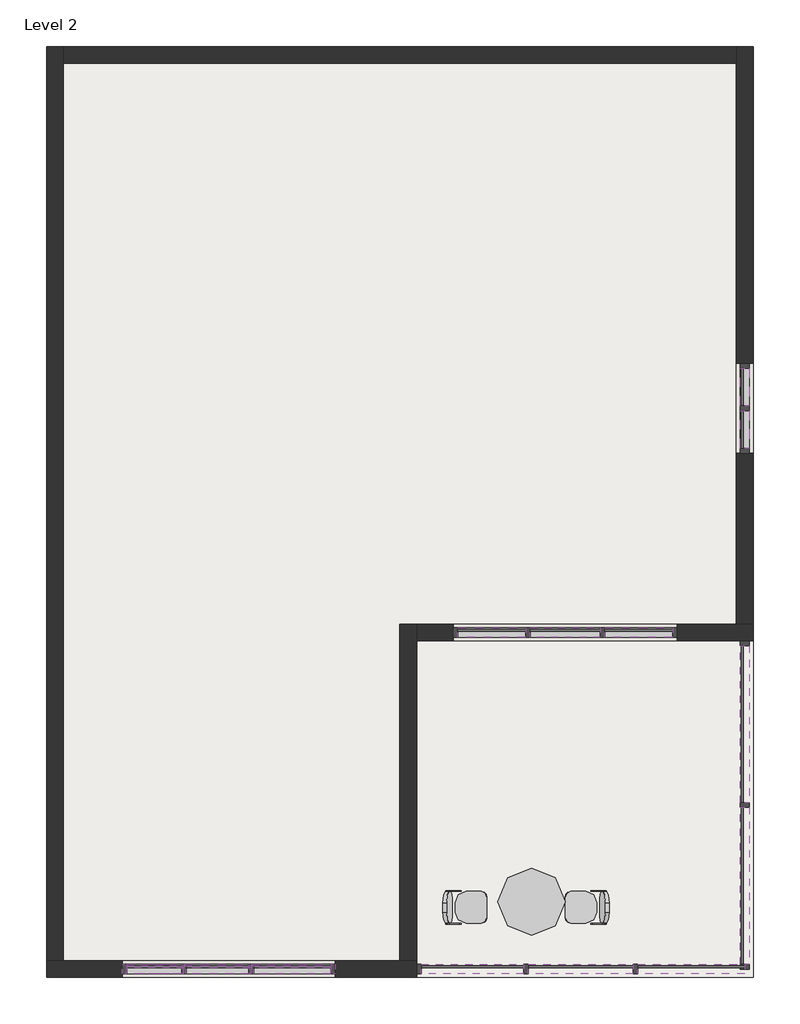
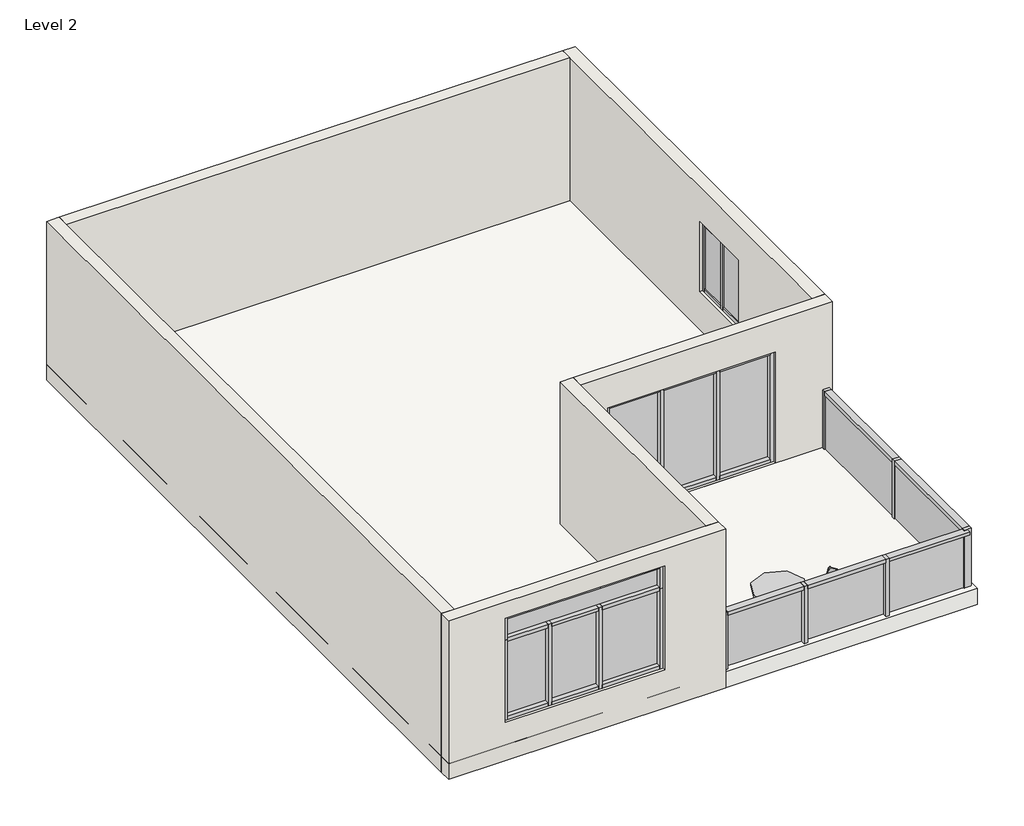
# One storey: 46 members, 14 plates, 6 walls, 3 furniture elements, 1 roof.
"""IFC4 building model written with IfcOpenShell, lengths in millimetres."""

from ifc_helpers import new_model, si_unit, frame, origin, place, context, project, spatial, polyline, outline, extrude, faceted_brep, transform, mapped, element, save
from components import furniture_eb3a3c23, furniture_ec754799, member_194e59d8, member_ff82125d, member_73c23c35, member_972adede, member_15823cb3, member_7b995701, member_7db1855a, member_7297827b, member_d2e7e466, member_3a0a7659, member_811bfb9a, member_697f972d, member_74e81316, member_78934672, member_cad56782, member_3e830f4e, member_0b7646a3, member_57611c17, member_d1dfe9dc, member_a36b500a, member_3bd69304, member_36d9a658, member_194437a1, member_a139046c, member_0767621a, member_3374d9b6, member_53538a1b, system_panel_glazed_d02f90d0, system_panel_glazed_14014958, system_panel_glazed_c1b5d4b5, system_panel_glazed_28e33a90, system_panel_glazed_a47c5a86, system_panel_glazed_f6d699fe, system_panel_glazed_2d65dcb0, system_panel_glazed_5a84bc76, system_panel_glazed_73858ddd, system_panel_glazed_ae745dbd, system_panel_glazed_f31d7781

model = new_model("IFC4")

# Units and contexts
model_context = context("Model", 3, world=origin())
ifc_project = project(units=[si_unit("LENGTHUNIT", "METRE", prefix="MILLI")], contexts=[model_context])

# Site, building, storey
site = spatial("IfcSite", under=ifc_project)
building = spatial("IfcBuilding", under=site)
storey = spatial("IfcBuildingStorey", under=building, Name="Level 2", Elevation=3048.0)

# Furniture
placement = place(None, origin())
furniture_shape = furniture_eb3a3c23(model_context)
element("IfcFurniture", 1, ObjectType="Seating-Auditorium : 18\" x 24\" x 30\"", at=placement, inside=storey, context=model_context, shape_type="MappedRepresentation", body=[
    mapped(furniture_shape, transform((-7671.1776869, -12175.0861758, 3048.0), x_axis=(0.0, 1.0, 0.0), y_axis=(-1.0, 0.0, 0.0), z_axis=(0.0, 0.0, 1.0))),
])
element("IfcFurniture", 2, ObjectType="Seating-Auditorium : 18\" x 24\" x 30\"", at=placement, inside=storey, context=model_context, shape_type="MappedRepresentation", body=[
    mapped(furniture_shape, transform((-9727.3285066, -11853.6304381, 3048.0), x_axis=(0.0, -1.0, 0.0), y_axis=(1.0, 0.0, 0.0), z_axis=(0.0, 0.0, 1.0))),
])
furniture_2_shape = furniture_ec754799(model_context)
element("IfcFurniture", 3, ObjectType="Table-Dining Round : 36\" Diameter", at=placement, inside=storey, context=model_context, shape_type="MappedRepresentation", body=[
    mapped(furniture_2_shape, transform((-8726.735064, -11753.2796184, 3048.0), x_axis=(1.0, 0.0, 0.0), y_axis=(0.0, 1.0, 0.0), z_axis=(0.0, 0.0, 1.0))),
])

# Members
member_shape = member_194e59d8(model_context)
element("IfcMember", 4, ObjectType="Rectangular Mullion : 2.5\" x 5\" rectangular", at=placement, inside=storey, context=model_context, shape_type="MappedRepresentation", body=[
    mapped(member_shape, transform((-7689.6030968, -8280.558307, 5481.9310998), x_axis=(0.0, 0.0, 1.0), y_axis=(0.0, -1.0, 0.0), z_axis=(1.0, 0.0, 0.0))),
])
member_2_shape = member_ff82125d(model_context)
element("IfcMember", 5, ObjectType="Rectangular Mullion : 2.5\" x 5\" rectangular", at=placement, inside=storey, context=model_context, shape_type="MappedRepresentation", body=[
    mapped(member_2_shape, transform((-8705.6030968, -8280.558307, 5481.9310998), x_axis=(0.0, 0.0, 1.0), y_axis=(0.0, -1.0, 0.0), z_axis=(1.0, 0.0, 0.0))),
])
element("IfcMember", 6, ObjectType="Rectangular Mullion : 2.5\" x 5\" rectangular", at=placement, inside=storey, context=model_context, shape_type="MappedRepresentation", body=[
    mapped(member_2_shape, transform((-6705.3530968, -8280.558307, 5481.9310998), x_axis=(0.0, 0.0, 1.0), y_axis=(0.0, -1.0, 0.0), z_axis=(1.0, 0.0, 0.0))),
])
element("IfcMember", 7, ObjectType="Rectangular Mullion : 2.5\" x 5\" rectangular", at=placement, inside=storey, context=model_context, shape_type="MappedRepresentation", body=[
    mapped(member_shape, transform((-8642.1030968, -8280.558307, 3352.8), x_axis=(0.0, 0.0, -1.0), y_axis=(0.0, -1.0, 0.0), z_axis=(-1.0, 0.0, 0.0))),
])
element("IfcMember", 8, ObjectType="Rectangular Mullion : 2.5\" x 5\" rectangular", at=placement, inside=storey, context=model_context, shape_type="MappedRepresentation", body=[
    mapped(member_2_shape, transform((-7626.1030968, -8280.558307, 3352.8), x_axis=(0.0, 0.0, -1.0), y_axis=(0.0, -1.0, 0.0), z_axis=(-1.0, 0.0, 0.0))),
])
element("IfcMember", 9, ObjectType="Rectangular Mullion : 2.5\" x 5\" rectangular", at=placement, inside=storey, context=model_context, shape_type="MappedRepresentation", body=[
    mapped(member_2_shape, transform((-9626.3530968, -8280.558307, 3352.8), x_axis=(0.0, 0.0, -1.0), y_axis=(0.0, -1.0, 0.0), z_axis=(-1.0, 0.0, 0.0))),
])
member_3_shape = member_73c23c35(model_context)
element("IfcMember", 10, ObjectType="Rectangular Mullion : 2.5\" x 5\" rectangular", at=placement, inside=storey, context=model_context, shape_type="MappedRepresentation", body=[
    mapped(member_3_shape, transform((-12433.0530968, -12852.558307, 5780.2418911), x_axis=(0.0, 0.0, 1.0), y_axis=(0.0, -1.0, 0.0), z_axis=(1.0, 0.0, 0.0))),
])
member_4_shape = member_972adede(model_context)
element("IfcMember", 11, ObjectType="Rectangular Mullion : 2.5\" x 5\" rectangular", at=placement, inside=storey, context=model_context, shape_type="MappedRepresentation", body=[
    mapped(member_4_shape, transform((-13347.4530968, -12852.558307, 5780.2418911), x_axis=(0.0, 0.0, 1.0), y_axis=(0.0, -1.0, 0.0), z_axis=(1.0, 0.0, 0.0))),
])
member_5_shape = member_15823cb3(model_context)
element("IfcMember", 12, ObjectType="Rectangular Mullion : 2.5\" x 5\" rectangular", at=placement, inside=storey, context=model_context, shape_type="MappedRepresentation", body=[
    mapped(member_5_shape, transform((-14185.6530968, -12852.558307, 5780.2418911), x_axis=(-1.0, 0.0, 0.0), y_axis=(0.0, -1.0, 0.0), z_axis=(0.0, 0.0, 1.0))),
])
member_6_shape = member_7b995701(model_context)
element("IfcMember", 13, ObjectType="Rectangular Mullion : 2.5\" x 5\" rectangular", at=placement, inside=storey, context=model_context, shape_type="MappedRepresentation", body=[
    mapped(member_6_shape, transform((-13379.2030968, -12852.558307, 5323.0418911), x_axis=(0.0, 0.0, 1.0), y_axis=(0.0, -1.0, 0.0), z_axis=(1.0, 0.0, 0.0))),
])
member_7_shape = member_7db1855a(model_context)
element("IfcMember", 14, ObjectType="Rectangular Mullion : 2.5\" x 5\" rectangular", at=placement, inside=storey, context=model_context, shape_type="MappedRepresentation", body=[
    mapped(member_7_shape, transform((-12464.8030968, -12852.558307, 5323.0418911), x_axis=(0.0, 0.0, 1.0), y_axis=(0.0, -1.0, 0.0), z_axis=(1.0, 0.0, 0.0))),
])
member_8_shape = member_7297827b(model_context)
element("IfcMember", 15, ObjectType="Rectangular Mullion : 2.5\" x 5\" rectangular", at=placement, inside=storey, context=model_context, shape_type="MappedRepresentation", body=[
    mapped(member_8_shape, transform((-13347.4530968, -12852.558307, 3783.7672722), x_axis=(1.0, 0.0, 0.0), y_axis=(0.0, -1.0, 0.0), z_axis=(0.0, 0.0, -1.0))),
])
element("IfcMember", 16, ObjectType="Rectangular Mullion : 2.5\" x 5\" rectangular", at=placement, inside=storey, context=model_context, shape_type="MappedRepresentation", body=[
    mapped(member_8_shape, transform((-12433.0530968, -12852.558307, 3783.7672722), x_axis=(1.0, 0.0, 0.0), y_axis=(0.0, -1.0, 0.0), z_axis=(0.0, 0.0, -1.0))),
])
member_9_shape = member_d2e7e466(model_context)
element("IfcMember", 17, ObjectType="Rectangular Mullion : 2.5\" x 5\" rectangular", at=placement, inside=storey, context=model_context, shape_type="MappedRepresentation", body=[
    mapped(member_9_shape, transform((-13315.7030968, -12852.558307, 3783.7672722), x_axis=(0.0, 0.0, -1.0), y_axis=(0.0, -1.0, 0.0), z_axis=(-1.0, 0.0, 0.0))),
])
member_10_shape = member_3a0a7659(model_context)
element("IfcMember", 18, ObjectType="Rectangular Mullion : 2.5\" x 5\" rectangular", at=placement, inside=storey, context=model_context, shape_type="MappedRepresentation", body=[
    mapped(member_10_shape, transform((-14122.1530968, -12852.558307, 3783.7672722), x_axis=(0.0, 0.0, -1.0), y_axis=(0.0, -1.0, 0.0), z_axis=(-1.0, 0.0, 0.0))),
])
member_11_shape = member_811bfb9a(model_context)
element("IfcMember", 19, ObjectType="Rectangular Mullion : 2.5\" x 5\" rectangular", at=placement, inside=storey, context=model_context, shape_type="MappedRepresentation", body=[
    mapped(member_11_shape, transform((-14185.6530968, -12852.558307, 5323.0418911), x_axis=(-1.0, 0.0, 0.0), y_axis=(0.0, -1.0, 0.0), z_axis=(0.0, 0.0, 1.0))),
])
member_12_shape = member_697f972d(model_context)
element("IfcMember", 20, ObjectType="Rectangular Mullion : 2.5\" x 5\" rectangular", at=placement, inside=storey, context=model_context, shape_type="MappedRepresentation", body=[
    mapped(member_12_shape, transform((-11353.5530968, -12852.558307, 5323.0418911), x_axis=(0.0, 0.0, 1.0), y_axis=(0.0, -1.0, 0.0), z_axis=(1.0, 0.0, 0.0))),
])
member_13_shape = member_74e81316(model_context)
element("IfcMember", 21, ObjectType="Rectangular Mullion : 2.5\" x 5\" rectangular", at=placement, inside=storey, context=model_context, shape_type="MappedRepresentation", body=[
    mapped(member_13_shape, transform((-11353.5530968, -12852.558307, 5780.2418911), x_axis=(0.0, 0.0, 1.0), y_axis=(0.0, -1.0, 0.0), z_axis=(1.0, 0.0, 0.0))),
])
member_14_shape = member_78934672(model_context)
element("IfcMember", 22, ObjectType="Rectangular Mullion : 2.5\" x 5\" rectangular", at=placement, inside=storey, context=model_context, shape_type="MappedRepresentation", body=[
    mapped(member_14_shape, transform((-12401.3030968, -12852.558307, 3783.7672722), x_axis=(0.0, 0.0, -1.0), y_axis=(0.0, -1.0, 0.0), z_axis=(-1.0, 0.0, 0.0))),
])
element("IfcMember", 23, ObjectType="Rectangular Mullion : 2.5\" x 5\" rectangular", at=placement, inside=storey, context=model_context, shape_type="MappedRepresentation", body=[
    mapped(member_5_shape, transform((-11290.0530968, -12852.558307, 5323.0418911), x_axis=(1.0, 0.0, 0.0), y_axis=(0.0, -1.0, 0.0), z_axis=(0.0, 0.0, -1.0))),
])
element("IfcMember", 24, ObjectType="Rectangular Mullion : 2.5\" x 5\" rectangular", at=placement, inside=storey, context=model_context, shape_type="MappedRepresentation", body=[
    mapped(member_11_shape, transform((-11290.0530968, -12852.558307, 3783.7672722), x_axis=(1.0, 0.0, 0.0), y_axis=(0.0, -1.0, 0.0), z_axis=(0.0, 0.0, -1.0))),
])
member_15_shape = member_cad56782(model_context)
element("IfcMember", 25, ObjectType="Rectangular Mullion : 2.5\" x 5\" rectangular", at=placement, inside=storey, context=model_context, shape_type="MappedRepresentation", body=[
    mapped(member_15_shape, transform((-8673.8530968, -8280.558307, 3352.8), x_axis=(1.0, 0.0, 0.0), y_axis=(0.0, -1.0, 0.0), z_axis=(0.0, 0.0, -1.0))),
])
element("IfcMember", 26, ObjectType="Rectangular Mullion : 2.5\" x 5\" rectangular", at=placement, inside=storey, context=model_context, shape_type="MappedRepresentation", body=[
    mapped(member_15_shape, transform((-7657.8530968, -8280.558307, 3352.8), x_axis=(1.0, 0.0, 0.0), y_axis=(0.0, -1.0, 0.0), z_axis=(0.0, 0.0, -1.0))),
])
member_16_shape = member_3e830f4e(model_context)
element("IfcMember", 27, ObjectType="Rectangular Mullion : 2.5\" x 5\" rectangular", at=placement, inside=storey, context=model_context, shape_type="MappedRepresentation", body=[
    mapped(member_16_shape, transform((-9689.8530968, -8280.558307, 5481.9310998), x_axis=(-1.0, 0.0, 0.0), y_axis=(0.0, -1.0, 0.0), z_axis=(0.0, 0.0, 1.0))),
])
element("IfcMember", 28, ObjectType="Rectangular Mullion : 2.5\" x 5\" rectangular", at=placement, inside=storey, context=model_context, shape_type="MappedRepresentation", body=[
    mapped(member_16_shape, transform((-6641.8530968, -8280.558307, 3352.8), x_axis=(1.0, 0.0, 0.0), y_axis=(0.0, -1.0, 0.0), z_axis=(0.0, 0.0, -1.0))),
])
member_17_shape = member_0b7646a3(model_context)
element("IfcMember", 29, ObjectType="Rectangular Mullion : 2.5\" x 5\" rectangular", at=placement, inside=storey, context=model_context, shape_type="MappedRepresentation", body=[
    mapped(member_17_shape, transform((-5727.4530968, -5264.308307, 5424.2538282), x_axis=(0.0, 0.0, 1.0), y_axis=(1.0, 0.0, 0.0), z_axis=(0.0, 1.0, 0.0))),
])
element("IfcMember", 30, ObjectType="Rectangular Mullion : 2.5\" x 5\" rectangular", at=placement, inside=storey, context=model_context, shape_type="MappedRepresentation", body=[
    mapped(member_17_shape, transform((-5727.4530968, -4686.458307, 5424.2538282), x_axis=(0.0, 0.0, 1.0), y_axis=(1.0, 0.0, 0.0), z_axis=(0.0, 1.0, 0.0))),
])
member_18_shape = member_57611c17(model_context)
element("IfcMember", 31, ObjectType="Rectangular Mullion : 2.5\" x 5\" rectangular", at=placement, inside=storey, context=model_context, shape_type="MappedRepresentation", body=[
    mapped(member_18_shape, transform((-5727.4530968, -5232.558307, 4082.4875559), x_axis=(0.0, 1.0, 0.0), y_axis=(1.0, 0.0, 0.0), z_axis=(0.0, 0.0, -1.0))),
])
element("IfcMember", 32, ObjectType="Rectangular Mullion : 2.5\" x 5\" rectangular", at=placement, inside=storey, context=model_context, shape_type="MappedRepresentation", body=[
    mapped(member_17_shape, transform((-5727.4530968, -5200.808307, 4082.4875559), x_axis=(0.0, 0.0, -1.0), y_axis=(1.0, 0.0, 0.0), z_axis=(0.0, -1.0, 0.0))),
])
element("IfcMember", 33, ObjectType="Rectangular Mullion : 2.5\" x 5\" rectangular", at=placement, inside=storey, context=model_context, shape_type="MappedRepresentation", body=[
    mapped(member_17_shape, transform((-5727.4530968, -5778.658307, 4082.4875559), x_axis=(0.0, 0.0, -1.0), y_axis=(1.0, 0.0, 0.0), z_axis=(0.0, -1.0, 0.0))),
])
member_19_shape = member_d1dfe9dc(model_context)
element("IfcMember", 34, ObjectType="Rectangular Mullion : 2.5\" x 5\" rectangular", at=placement, inside=storey, context=model_context, shape_type="MappedRepresentation", body=[
    mapped(member_19_shape, transform((-5727.4530968, -5842.158307, 5424.2538282), x_axis=(0.0, -1.0, 0.0), y_axis=(1.0, 0.0, 0.0), z_axis=(0.0, 0.0, 1.0))),
])
element("IfcMember", 35, ObjectType="Rectangular Mullion : 2.5\" x 5\" rectangular", at=placement, inside=storey, context=model_context, shape_type="MappedRepresentation", body=[
    mapped(member_19_shape, transform((-5727.4530968, -4622.958307, 4082.4875559), x_axis=(0.0, 1.0, 0.0), y_axis=(1.0, 0.0, 0.0), z_axis=(0.0, 0.0, -1.0))),
])
member_20_shape = member_a36b500a(model_context)
element("IfcMember", 36, ObjectType="Rectangular Mullion : 2.5\" x 5\" rectangular", at=placement, inside=storey, context=model_context, shape_type="MappedRepresentation", body=[
    mapped(member_20_shape, transform((-8731.0030968, -12852.558307, 4454.4174829), x_axis=(0.0, 0.0, 1.0), y_axis=(0.0, -1.0, 0.0), z_axis=(1.0, 0.0, 0.0))),
])
member_21_shape = member_3bd69304(model_context)
element("IfcMember", 37, ObjectType="Rectangular Mullion : 2.5\" x 5\" rectangular", at=placement, inside=storey, context=model_context, shape_type="MappedRepresentation", body=[
    mapped(member_21_shape, transform((-8699.2530968, -12852.558307, 3048.0), x_axis=(1.0, 0.0, 0.0), y_axis=(0.0, -1.0, 0.0), z_axis=(0.0, 0.0, -1.0))),
])
element("IfcMember", 38, ObjectType="Rectangular Mullion : 2.5\" x 5\" rectangular", at=placement, inside=storey, context=model_context, shape_type="MappedRepresentation", body=[
    mapped(member_21_shape, transform((-7213.3530968, -12852.558307, 3048.0), x_axis=(1.0, 0.0, 0.0), y_axis=(0.0, -1.0, 0.0), z_axis=(0.0, 0.0, -1.0))),
])
element("IfcMember", 39, ObjectType="Rectangular Mullion : 2.5\" x 5\" rectangular", at=placement, inside=storey, context=model_context, shape_type="MappedRepresentation", body=[
    mapped(member_20_shape, transform((-10121.6530968, -12852.558307, 3048.0), x_axis=(0.0, 0.0, -1.0), y_axis=(0.0, -1.0, 0.0), z_axis=(-1.0, 0.0, 0.0))),
])
member_22_shape = member_36d9a658(model_context)
element("IfcMember", 40, ObjectType="Rectangular Mullion : 2.5\" x 5\" rectangular", at=placement, inside=storey, context=model_context, shape_type="MappedRepresentation", body=[
    mapped(member_22_shape, transform((-10185.1530968, -12852.558307, 4454.4174829), x_axis=(-1.0, 0.0, 0.0), y_axis=(0.0, -1.0, 0.0), z_axis=(0.0, 0.0, 1.0))),
])
member_23_shape = member_194437a1(model_context)
element("IfcMember", 41, ObjectType="Rectangular Mullion : 2.5\" x 5\" rectangular", at=placement, inside=storey, context=model_context, shape_type="MappedRepresentation", body=[
    mapped(member_23_shape, transform((-7245.1030968, -12852.558307, 4454.4174829), x_axis=(0.0, 0.0, 1.0), y_axis=(0.0, -1.0, 0.0), z_axis=(1.0, 0.0, 0.0))),
])
member_24_shape = member_a139046c(model_context)
element("IfcMember", 42, ObjectType="Rectangular Mullion : 2.5\" x 5\" rectangular", at=placement, inside=storey, context=model_context, shape_type="MappedRepresentation", body=[
    mapped(member_24_shape, transform((-5727.4530968, -12852.558307, 4454.4174829), x_axis=(0.0, 0.0, 1.0), y_axis=(0.0, -1.0, 0.0), z_axis=(1.0, 0.0, 0.0))),
])
element("IfcMember", 43, ObjectType="Rectangular Mullion : 2.5\" x 5\" rectangular", at=placement, inside=storey, context=model_context, shape_type="MappedRepresentation", body=[
    mapped(member_24_shape, transform((-7181.6030968, -12852.558307, 3048.0), x_axis=(0.0, 0.0, -1.0), y_axis=(0.0, -1.0, 0.0), z_axis=(-1.0, 0.0, 0.0))),
])
element("IfcMember", 44, ObjectType="Rectangular Mullion : 2.5\" x 5\" rectangular", at=placement, inside=storey, context=model_context, shape_type="MappedRepresentation", body=[
    mapped(member_23_shape, transform((-8667.5030968, -12852.558307, 3048.0), x_axis=(0.0, 0.0, -1.0), y_axis=(0.0, -1.0, 0.0), z_axis=(-1.0, 0.0, 0.0))),
])
member_25_shape = member_0767621a(model_context)
element("IfcMember", 45, ObjectType="Rectangular Mullion : 2.5\" x 5\" rectangular", at=placement, inside=storey, context=model_context, shape_type="MappedRepresentation", body=[
    mapped(member_25_shape, transform((-5727.4530968, -10623.708307, 3048.0), x_axis=(0.0, 1.0, 0.0), y_axis=(1.0, 0.0, 0.0), z_axis=(0.0, 0.0, -1.0))),
])
member_26_shape = member_3374d9b6(model_context)
element("IfcMember", 46, ObjectType="Rectangular Mullion : 2.5\" x 5\" rectangular", at=placement, inside=storey, context=model_context, shape_type="MappedRepresentation", body=[
    mapped(member_26_shape, transform((-5727.4530968, -10655.458307, 4463.2614699), x_axis=(0.0, 0.0, 1.0), y_axis=(1.0, 0.0, 0.0), z_axis=(0.0, 1.0, 0.0))),
])
element("IfcMember", 47, ObjectType="Rectangular Mullion : 2.5\" x 5\" rectangular", at=placement, inside=storey, context=model_context, shape_type="MappedRepresentation", body=[
    mapped(member_26_shape, transform((-5727.4530968, -8458.358307, 4463.2614699), x_axis=(0.0, 0.0, 1.0), y_axis=(1.0, 0.0, 0.0), z_axis=(0.0, 1.0, 0.0))),
])
member_27_shape = member_53538a1b(model_context)
element("IfcMember", 48, ObjectType="Rectangular Mullion : 2.5\" x 5\" rectangular", at=placement, inside=storey, context=model_context, shape_type="MappedRepresentation", body=[
    mapped(member_27_shape, transform((-5727.4530968, -12852.558307, 4463.2614699), x_axis=(0.0, -1.0, 0.0), y_axis=(1.0, 0.0, 0.0), z_axis=(0.0, 0.0, 1.0))),
])
element("IfcMember", 49, ObjectType="Rectangular Mullion : 2.5\" x 5\" rectangular", at=placement, inside=storey, context=model_context, shape_type="MappedRepresentation", body=[
    mapped(member_27_shape, transform((-5727.4530968, -8394.858307, 3048.0), x_axis=(0.0, 1.0, 0.0), y_axis=(1.0, 0.0, 0.0), z_axis=(0.0, 0.0, -1.0))),
])

# Plates
system_panel_glazed_shape = system_panel_glazed_d02f90d0(model_context)
element("IfcPlate", 50, ObjectType="System Panel : Glazed", at=placement, inside=storey, context=model_context, shape_type="MappedRepresentation", body=[
    mapped(system_panel_glazed_shape, transform((-13750.6780968, -12852.558307, 3847.2672722), x_axis=(1.0, 0.0, 0.0), y_axis=(0.0, 1.0, 0.0), z_axis=(0.0, 0.0, 1.0))),
])
system_panel_glazed_2_shape = system_panel_glazed_14014958(model_context)
element("IfcPlate", 51, ObjectType="System Panel : Glazed", at=placement, inside=storey, context=model_context, shape_type="MappedRepresentation", body=[
    mapped(system_panel_glazed_2_shape, transform((-12890.2530968, -12852.558307, 3847.2672722), x_axis=(1.0, 0.0, 0.0), y_axis=(0.0, 1.0, 0.0), z_axis=(0.0, 0.0, 1.0))),
])
system_panel_glazed_3_shape = system_panel_glazed_c1b5d4b5(model_context)
element("IfcPlate", 52, ObjectType="System Panel : Glazed", at=placement, inside=storey, context=model_context, shape_type="MappedRepresentation", body=[
    mapped(system_panel_glazed_3_shape, transform((-12737.8530968, -12852.558307, 5354.7918911), x_axis=(1.0, 0.0, 0.0), y_axis=(0.0, 1.0, 0.0), z_axis=(0.0, 0.0, 1.0))),
])
system_panel_glazed_4_shape = system_panel_glazed_28e33a90(model_context)
element("IfcPlate", 53, ObjectType="System Panel : Glazed", at=placement, inside=storey, context=model_context, shape_type="MappedRepresentation", body=[
    mapped(system_panel_glazed_4_shape, transform((-11877.4280968, -12852.558307, 3847.2672722), x_axis=(1.0, 0.0, 0.0), y_axis=(0.0, 1.0, 0.0), z_axis=(0.0, 0.0, 1.0))),
])
system_panel_glazed_5_shape = system_panel_glazed_a47c5a86(model_context)
element("IfcPlate", 54, ObjectType="System Panel : Glazed", at=placement, inside=storey, context=model_context, shape_type="MappedRepresentation", body=[
    mapped(system_panel_glazed_5_shape, transform((-9165.9780968, -8280.558307, 3416.3), x_axis=(1.0, 0.0, 0.0), y_axis=(0.0, 1.0, 0.0), z_axis=(0.0, 0.0, 1.0))),
])
element("IfcPlate", 55, ObjectType="System Panel : Glazed", at=placement, inside=storey, context=model_context, shape_type="MappedRepresentation", body=[
    mapped(system_panel_glazed_5_shape, transform((-7165.7280968, -8280.558307, 3416.3), x_axis=(1.0, 0.0, 0.0), y_axis=(0.0, 1.0, 0.0), z_axis=(0.0, 0.0, 1.0))),
])
system_panel_glazed_6_shape = system_panel_glazed_f6d699fe(model_context)
element("IfcPlate", 56, ObjectType="System Panel : Glazed", at=placement, inside=storey, context=model_context, shape_type="MappedRepresentation", body=[
    mapped(system_panel_glazed_6_shape, transform((-8165.8530968, -8280.558307, 3416.3), x_axis=(1.0, 0.0, 0.0), y_axis=(0.0, 1.0, 0.0), z_axis=(0.0, 0.0, 1.0))),
])
system_panel_glazed_7_shape = system_panel_glazed_2d65dcb0(model_context)
element("IfcPlate", 57, ObjectType="System Panel : Glazed", at=placement, inside=storey, context=model_context, shape_type="MappedRepresentation", body=[
    mapped(system_panel_glazed_7_shape, transform((-5727.4530968, -5521.483307, 4145.9875559), x_axis=(0.0, 1.0, 0.0), y_axis=(-1.0, 0.0, 0.0), z_axis=(0.0, 0.0, 1.0))),
])
element("IfcPlate", 58, ObjectType="System Panel : Glazed", at=placement, inside=storey, context=model_context, shape_type="MappedRepresentation", body=[
    mapped(system_panel_glazed_7_shape, transform((-5727.4530968, -4943.633307, 4145.9875559), x_axis=(0.0, 1.0, 0.0), y_axis=(-1.0, 0.0, 0.0), z_axis=(0.0, 0.0, 1.0))),
])
system_panel_glazed_8_shape = system_panel_glazed_5a84bc76(model_context)
element("IfcPlate", 59, ObjectType="System Panel : Glazed", at=placement, inside=storey, context=model_context, shape_type="MappedRepresentation", body=[
    mapped(system_panel_glazed_8_shape, transform((-9426.3280968, -12852.558307, 3111.5), x_axis=(1.0, 0.0, 0.0), y_axis=(0.0, 1.0, 0.0), z_axis=(0.0, 0.0, 1.0))),
])
system_panel_glazed_9_shape = system_panel_glazed_73858ddd(model_context)
element("IfcPlate", 60, ObjectType="System Panel : Glazed", at=placement, inside=storey, context=model_context, shape_type="MappedRepresentation", body=[
    mapped(system_panel_glazed_9_shape, transform((-6454.5280968, -12852.558307, 3111.5), x_axis=(1.0, 0.0, 0.0), y_axis=(0.0, 1.0, 0.0), z_axis=(0.0, 0.0, 1.0))),
])
system_panel_glazed_10_shape = system_panel_glazed_ae745dbd(model_context)
element("IfcPlate", 61, ObjectType="System Panel : Glazed", at=placement, inside=storey, context=model_context, shape_type="MappedRepresentation", body=[
    mapped(system_panel_glazed_10_shape, transform((-7956.3030968, -12852.558307, 3111.5), x_axis=(1.0, 0.0, 0.0), y_axis=(0.0, 1.0, 0.0), z_axis=(0.0, 0.0, 1.0))),
])
system_panel_glazed_11_shape = system_panel_glazed_f31d7781(model_context)
element("IfcPlate", 62, ObjectType="System Panel : Glazed", at=placement, inside=storey, context=model_context, shape_type="MappedRepresentation", body=[
    mapped(system_panel_glazed_11_shape, transform((-5727.4530968, -11722.258307, 3048.0), x_axis=(0.0, 1.0, 0.0), y_axis=(-1.0, 0.0, 0.0), z_axis=(0.0, 0.0, 1.0))),
])
element("IfcPlate", 63, ObjectType="System Panel : Glazed", at=placement, inside=storey, context=model_context, shape_type="MappedRepresentation", body=[
    mapped(system_panel_glazed_11_shape, transform((-5727.4530968, -9525.158307, 3048.0), x_axis=(0.0, 1.0, 0.0), y_axis=(-1.0, 0.0, 0.0), z_axis=(0.0, 0.0, 1.0))),
])

# Roof
element("IfcRoof", 64, ObjectType="Generic - 12\"", at=placement, inside=storey, context=model_context, shape_type="SweptSolid", body=[
    extrude(outline(polyline([(-15214.3530968, -317.658307), (-5613.1530968, -317.658307), (-5613.1530968, -12966.858307), (-15214.3530968, -12966.858307), (-15214.3530968, -317.658307)])), frame((0.0, 0.0, 3048.0), z_axis=(0.0, 0.0, 1.0), x_axis=(1.0, 0.0, 0.0)), (0.0, 0.0, 1.0), 304.8),
])

# Walls
element("IfcWall", 65, ObjectType="9\"", at=placement, inside=storey, context=model_context, shape_type="Brep", body=[
    faceted_brep([(-15214.3530968, -12966.858307, 3048.0), (-10185.1530968, -12966.858307, 3048.0), (-10185.1530968, -12966.858307, 6096.0), (-15214.3530968, -12966.858307, 6096.0), (-14185.6530968, -12966.858307, 3783.7672722), (-14185.6530968, -12966.858307, 5780.2418911), (-11290.0530968, -12966.858307, 5780.2418911), (-11290.0530968, -12966.858307, 3783.7672722), (-10185.1530968, -12738.258307, 3048.0), (-10413.7530968, -12738.258307, 3048.0), (-14985.7530968, -12738.258307, 3048.0), (-15214.3530968, -12738.258307, 3048.0), (-15214.3530968, -12738.258307, 6096.0), (-14985.7530968, -12738.258307, 6096.0), (-10413.7530968, -12738.258307, 6096.0), (-10185.1530968, -12738.258307, 6096.0), (-14185.6530968, -12738.258307, 5780.2418911), (-14185.6530968, -12738.258307, 3783.7672722), (-11290.0530968, -12738.258307, 3783.7672722), (-11290.0530968, -12738.258307, 5780.2418911)], [[[0, 1, 2, 3], [4, 5, 6, 7]], [[8, 9, 10, 11, 12, 13, 14, 15], [16, 17, 18, 19]], [[1, 0, 11, 10, 9, 8]], [[3, 2, 15, 14, 13, 12]], [[2, 1, 8, 15]], [[0, 3, 12, 11]], [[4, 17, 16, 5]], [[5, 16, 19, 6]], [[6, 19, 18, 7]], [[17, 4, 7, 18]]]),
])
element("IfcWall", 66, ObjectType="9\"", at=placement, inside=storey, context=model_context, shape_type="Brep", body=[
    faceted_brep([(-10185.1530968, -12738.258307, 3048.0), (-10185.1530968, -8394.858307, 3048.0), (-10185.1530968, -8166.258307, 3048.0), (-10185.1530968, -8166.258307, 6096.0), (-10185.1530968, -8394.858307, 6096.0), (-10185.1530968, -12738.258307, 6096.0), (-10413.7530968, -12738.258307, 3048.0), (-10413.7530968, -12738.258307, 6096.0), (-10413.7530968, -8166.258307, 6096.0), (-10413.7530968, -8166.258307, 3048.0)], [[[0, 1, 2, 3, 4, 5]], [[6, 7, 8, 9]], [[2, 1, 0, 6, 9]], [[5, 4, 3, 8, 7]], [[0, 5, 7, 6]], [[3, 2, 9, 8]]]),
])
element("IfcWall", 67, ObjectType="9\"", at=placement, inside=storey, context=model_context, shape_type="Brep", body=[
    faceted_brep([(-10185.1530968, -8394.858307, 3048.0), (-5613.1530968, -8394.858307, 3048.0), (-5613.1530968, -8394.858307, 6096.0), (-10185.1530968, -8394.858307, 6096.0), (-9689.8530968, -8394.858307, 3352.8), (-9689.8530968, -8394.858307, 5481.9310998), (-6641.8530968, -8394.858307, 5481.9310998), (-6641.8530968, -8394.858307, 3352.8), (-5613.1530968, -8166.258307, 3048.0), (-5841.7530968, -8166.258307, 3048.0), (-10185.1530968, -8166.258307, 3048.0), (-10185.1530968, -8166.258307, 6096.0), (-5841.7530968, -8166.258307, 6096.0), (-5613.1530968, -8166.258307, 6096.0), (-9689.8530968, -8166.258307, 5481.9310998), (-9689.8530968, -8166.258307, 3352.8), (-6641.8530968, -8166.258307, 3352.8), (-6641.8530968, -8166.258307, 5481.9310998)], [[[0, 1, 2, 3], [4, 5, 6, 7]], [[8, 9, 10, 11, 12, 13], [14, 15, 16, 17]], [[1, 0, 10, 9, 8]], [[3, 2, 13, 12, 11]], [[0, 3, 11, 10]], [[2, 1, 8, 13]], [[4, 15, 14, 5]], [[5, 14, 17, 6]], [[6, 17, 16, 7]], [[15, 4, 7, 16]]]),
])
element("IfcWall", 68, ObjectType="9\"", at=placement, inside=storey, context=model_context, shape_type="Brep", body=[
    faceted_brep([(-5613.1530968, -8166.258307, 3048.0), (-5613.1530968, -317.658307, 3048.0), (-5613.1530968, -317.658307, 6096.0), (-5613.1530968, -8166.258307, 6096.0), (-5613.1530968, -5842.158307, 4082.4875559), (-5613.1530968, -5842.158307, 5424.2538282), (-5613.1530968, -4622.958307, 5424.2538282), (-5613.1530968, -4622.958307, 4082.4875559), (-5841.7530968, -317.658307, 3048.0), (-5841.7530968, -546.258307, 3048.0), (-5841.7530968, -8166.258307, 3048.0), (-5841.7530968, -8166.258307, 6096.0), (-5841.7530968, -546.258307, 6096.0), (-5841.7530968, -317.658307, 6096.0), (-5841.7530968, -5842.158307, 5424.2538282), (-5841.7530968, -5842.158307, 4082.4875559), (-5841.7530968, -4622.958307, 4082.4875559), (-5841.7530968, -4622.958307, 5424.2538282)], [[[0, 1, 2, 3], [4, 5, 6, 7]], [[8, 9, 10, 11, 12, 13], [14, 15, 16, 17]], [[1, 0, 10, 9, 8]], [[3, 2, 13, 12, 11]], [[0, 3, 11, 10]], [[2, 1, 8, 13]], [[4, 15, 14, 5]], [[5, 14, 17, 6]], [[6, 17, 16, 7]], [[15, 4, 7, 16]]]),
])
element("IfcWall", 69, ObjectType="9\"", at=placement, inside=storey, context=model_context, shape_type="Brep", body=[
    faceted_brep([(-15214.3530968, -317.658307, 3048.0), (-15214.3530968, -12738.258307, 3048.0), (-15214.3530968, -12738.258307, 6096.0), (-15214.3530968, -317.658307, 6096.0), (-14985.7530968, -317.658307, 3048.0), (-14985.7530968, -317.658307, 6096.0), (-14985.7530968, -546.258307, 6096.0), (-14985.7530968, -12738.258307, 6096.0), (-14985.7530968, -12738.258307, 3048.0), (-14985.7530968, -546.258307, 3048.0)], [[[0, 1, 2, 3]], [[4, 5, 6, 7, 8, 9]], [[1, 0, 4, 9, 8]], [[3, 2, 7, 6, 5]], [[2, 1, 8, 7]], [[0, 3, 5, 4]]]),
])
element("IfcWall", 70, ObjectType="9\"", at=placement, inside=storey, context=model_context, shape_type="SweptSolid", body=[
    extrude(outline(polyline([(-5841.7530968, -546.258307), (-14985.7530968, -546.258307), (-14985.7530968, -317.658307), (-5841.7530968, -317.658307), (-5841.7530968, -546.258307)])), frame((0.0, 0.0, 3048.0), z_axis=(0.0, 0.0, 1.0), x_axis=(1.0, 0.0, 0.0)), (0.0, 0.0, 1.0), 3048.0),
])

save(model, "model.ifc")

# Revit data of these elements
# Type "Seating-Auditorium : 18\" x 24\" x 30\""
#   Assembly Code = "E2020200"
#   Seat Material = Linen, Beige
#   Frame Material = Steel, Paint Finish, Dark Gray, Matte
#   Default Elevation = 0
# Type "Table-Dining Round : 36\" Diameter"
#   Assembly Code = "E2020200"
#   Diameter = 3' - 0"
#   Height = 2' - 6"
#   Base Material = Pine
#   Top Material = Laminate, Linen, Matte
#   Default Elevation = 0
# Type "Rectangular Mullion : 2.5\" x 5\" rectangular"
#   built-in parameter 1007304 = 0.416667 (stored number, unit not read)
#   built-in parameter 1007301 = 0.104167 (stored number, unit not read)
#   built-in parameter 1007300 = 0.104167 (stored number, unit not read)
# Type "System Panel : Glazed"
#   Construction Type Id = "GSP4R"
#   Analytic Construction = "1/8 in Pilkington single glazing"
#   Visual Light Transmittance = 0.9
#   Solar Heat Gain Coefficient = 0.86
#   Heat Transfer Coefficient (U) = 1.18115 BTU/(h·ft²·°F)
#   Define Thermal Properties by = 1
# Type "Generic - 12\""
#   Assembly Code = "B1020"
#   Layers, outside or top first: 1' - 0" no material (function 1)
# Type "9\""
#   Assembly Code = "B2010"
#   Layers, outside or top first: 0' - 9" no material (function 1)
# Elements 1, 2 (IfcFurniture, "Seating-Auditorium : 18\" x 24\" x 30\"")
#   Phase Created = New Construction
#   Materials on its faces: "Steel, Paint Finish, Dark Gray, Matte", "Linen, Beige"
# Element 3 (IfcFurniture, "Table-Dining Round : 36\" Diameter")
#   Phase Created = New Construction
#   Materials on its faces: "Pine", "Laminate, Linen, Matte"
# Elements 4, 5, 6, 7, 8, 9, 10, 11, 12, 13, 14, 15, 16, 17, 18, 19, 20, 21, 22, 23, 24, 25, 26, 27, 28, 29, 30, 31, 32, 33, 34, 35, 36, 37, 38, 39, 40, 41, 42, 43, 44, 45, 46, 47, 48, 49 (IfcMember, "Rectangular Mullion : 2.5\" x 5\" rectangular")
#   Phase Created = New Construction
#   Materials on its faces: "Aluminum"
# Elements 50, 51, 52, 53, 54, 55, 56, 57, 58, 59, 60, 61, 62, 63 (IfcPlate, "System Panel : Glazed")
#   Phase Created = New Construction
#   Materials on its faces: "Glass"
# Element 64 (IfcRoof, "Generic - 12\"")
#   built-in parameter 1001705 = 11 (stored number, unit not read)
#   built-in parameter 1001710 = 33615
#   Phase Created = New Construction
#   Materials on its faces: "Default Roof"
# Elements 65, 66, 67, 68, 69, 70 (IfcWall, "9\"")
#   Top Offset = 0' - 0"
#   Base Offset = 0' - 0"
#   Unconnected Height = 10' - 0"
#   wall height = 10' - 0"
#   Phase Created = New Construction
#   Base Constraint = Level 2
#   Materials on its faces: "Default Wall"
# Materials
#   "Linen, Beige": class "Textile", colour RGB 249 239 230, transparency 0, Description = "Linen, beige", Cost = 0
#   "Steel, Paint Finish, Dark Gray, Matte": class "Metal", colour RGB 0 0 0, transparency 0, Description = "Steel, paint finish, dark gray, matte", Cost = 0
#   "Pine": class "Wood", colour RGB 223 192 134, transparency 0, Description = "Pinus Echinata", Cost = 0
#   "Laminate, Linen, Matte": class "Plastic", colour RGB 249 239 230, transparency 0, Description = "Plastic Laminate - Linen, Matte", Cost = 0
#   "Aluminum": class "Metal", colour RGB 247 247 247, transparency 0, Description = "Aluminum 6061", Cost = 0
#   "Glass": class "Glass", colour RGB 0 128 192, transparency 0.75, Description = "Soda Lime Glass", Cost = 0
#   "Default Roof": colour RGB 88 101 114, transparency 0, Cost = 0
#   "Default Wall": colour RGB 128 128 128, transparency 0, Cost = 0
